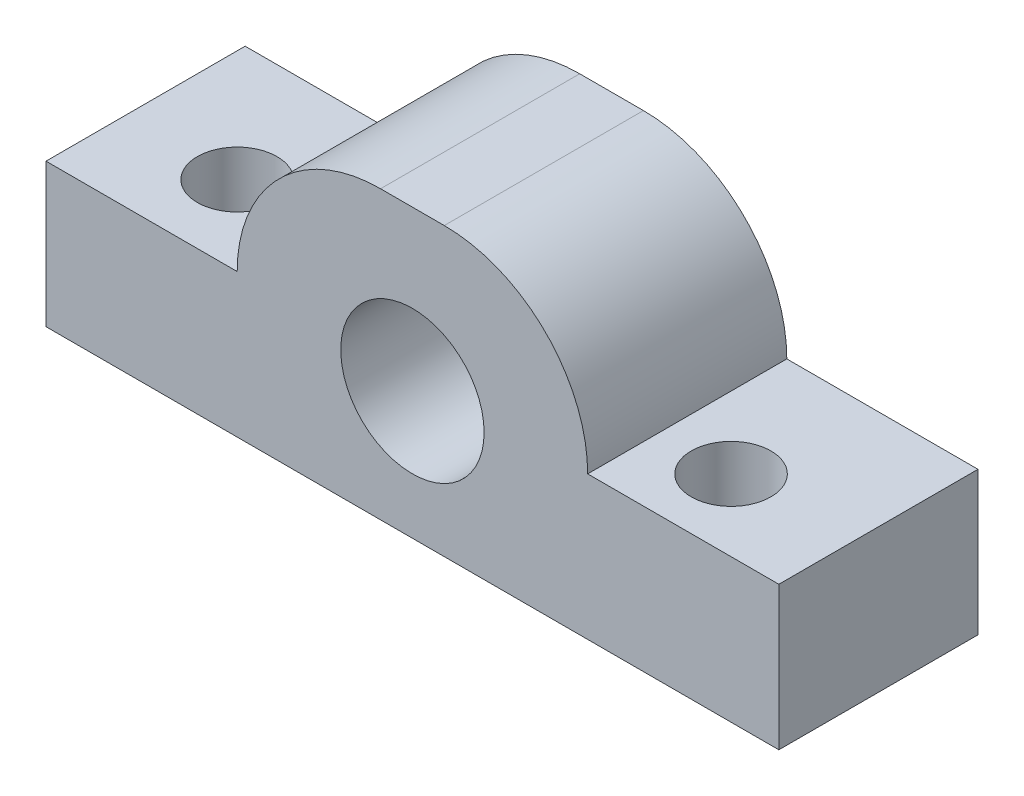
ISO-10303-21;
HEADER;
FILE_DESCRIPTION(('STEP AP214'),'2;1');
FILE_NAME('part.step','',(''),(''),'','','');
FILE_SCHEMA(('AUTOMOTIVE_DESIGN { 1 0 10303 214 1 1 1 1 }'));
ENDSEC;
DATA;
#1=APPLICATION_CONTEXT('core data for automotive mechanical design processes');
#2=APPLICATION_PROTOCOL_DEFINITION('international standard','automotive_design',2000,#1);
#3=PRODUCT_CONTEXT('',#1,'mechanical');
#4=PRODUCT('Part','Part','',(#3));
#5=PRODUCT_RELATED_PRODUCT_CATEGORY('part','',(#4));
#6=PRODUCT_DEFINITION_FORMATION('','',#4);
#7=PRODUCT_DEFINITION_CONTEXT('part definition',#1,'design');
#8=PRODUCT_DEFINITION('design','',#6,#7);
#9=PRODUCT_DEFINITION_SHAPE('','',#8);
#10=(LENGTH_UNIT() NAMED_UNIT(*) SI_UNIT(.MILLI.,.METRE.));
#11=(NAMED_UNIT(*) PLANE_ANGLE_UNIT() SI_UNIT($,.RADIAN.));
#12=(NAMED_UNIT(*) SI_UNIT($,.STERADIAN.) SOLID_ANGLE_UNIT());
#13=UNCERTAINTY_MEASURE_WITH_UNIT(LENGTH_MEASURE(1.E-05),#10,'distance_accuracy_value','');
#14=(GEOMETRIC_REPRESENTATION_CONTEXT(3) GLOBAL_UNCERTAINTY_ASSIGNED_CONTEXT((#13)) GLOBAL_UNIT_ASSIGNED_CONTEXT((#10,
#11,#12)) REPRESENTATION_CONTEXT('',''));
#15=CARTESIAN_POINT('',(0.,0.,0.));
#16=DIRECTION('',(0.,0.,1.));
#17=DIRECTION('',(1.,0.,0.));
#18=AXIS2_PLACEMENT_3D('',#15,#16,#17);
#19=CARTESIAN_POINT('',(-4.,18.,12.5));
#20=DIRECTION('',(0.,0.,-1.));
#21=DIRECTION('',(-1.,0.,0.));
#22=AXIS2_PLACEMENT_3D('',#19,#20,#21);
#23=PLANE('',#22);
#24=DIRECTION('',(0.,-1.,0.));
#25=VECTOR('',#24,1.);
#26=CARTESIAN_POINT('',(-46.,0.,12.5));
#27=LINE('',#26,#25);
#28=CARTESIAN_POINT('',(-46.,18.,12.5));
#29=VERTEX_POINT('',#28);
#30=CARTESIAN_POINT('',(-46.,0.,12.5));
#31=VERTEX_POINT('',#30);
#32=EDGE_CURVE('E151',#29,#31,#27,.T.);
#33=ORIENTED_EDGE('',*,*,#32,.T.);
#34=DIRECTION('',(1.,0.,0.));
#35=VECTOR('',#34,1.);
#36=CARTESIAN_POINT('',(46.,0.,12.5));
#37=LINE('',#36,#35);
#38=CARTESIAN_POINT('',(46.,0.,12.5));
#39=VERTEX_POINT('',#38);
#40=EDGE_CURVE('E97',#31,#39,#37,.T.);
#41=ORIENTED_EDGE('',*,*,#40,.T.);
#42=DIRECTION('',(0.,1.,0.));
#43=VECTOR('',#42,1.);
#44=CARTESIAN_POINT('',(46.,0.,12.5));
#45=LINE('',#44,#43);
#46=CARTESIAN_POINT('',(46.,18.,12.5));
#47=VERTEX_POINT('',#46);
#48=EDGE_CURVE('E167',#39,#47,#45,.T.);
#49=ORIENTED_EDGE('',*,*,#48,.T.);
#50=DIRECTION('',(-1.,0.,0.));
#51=VECTOR('',#50,1.);
#52=CARTESIAN_POINT('',(46.,18.,12.5));
#53=LINE('',#52,#51);
#54=CARTESIAN_POINT('',(22.,18.,12.5));
#55=VERTEX_POINT('',#54);
#56=EDGE_CURVE('E179',#47,#55,#53,.T.);
#57=ORIENTED_EDGE('',*,*,#56,.T.);
#58=CARTESIAN_POINT('',(4.,18.,12.5));
#59=DIRECTION('',(0.,0.,1.));
#60=DIRECTION('',(1.,0.,0.));
#61=AXIS2_PLACEMENT_3D('',#58,#59,#60);
#62=CIRCLE('',#61,18.);
#63=CARTESIAN_POINT('',(4.,36.,12.5));
#64=VERTEX_POINT('',#63);
#65=EDGE_CURVE('E120',#55,#64,#62,.T.);
#66=ORIENTED_EDGE('',*,*,#65,.T.);
#67=DIRECTION('',(-1.,0.,0.));
#68=VECTOR('',#67,1.);
#69=CARTESIAN_POINT('',(-4.,36.,12.5));
#70=LINE('',#69,#68);
#71=CARTESIAN_POINT('',(-4.,36.,12.5));
#72=VERTEX_POINT('',#71);
#73=EDGE_CURVE('E115',#64,#72,#70,.T.);
#74=ORIENTED_EDGE('',*,*,#73,.T.);
#75=CARTESIAN_POINT('',(-4.,18.,12.5));
#76=DIRECTION('',(0.,0.,1.));
#77=DIRECTION('',(-1.,0.,0.));
#78=AXIS2_PLACEMENT_3D('',#75,#76,#77);
#79=CIRCLE('',#78,18.);
#80=CARTESIAN_POINT('',(-22.,18.,12.5));
#81=VERTEX_POINT('',#80);
#82=EDGE_CURVE('E119',#72,#81,#79,.T.);
#83=ORIENTED_EDGE('',*,*,#82,.T.);
#84=DIRECTION('',(-1.,0.,0.));
#85=VECTOR('',#84,1.);
#86=CARTESIAN_POINT('',(-46.,18.,12.5));
#87=LINE('',#86,#85);
#88=EDGE_CURVE('E57',#81,#29,#87,.T.);
#89=ORIENTED_EDGE('',*,*,#88,.T.);
#90=EDGE_LOOP('',(#33,#41,#49,#57,#66,#74,#83,#89));
#91=FACE_BOUND('',#90,.T.);
#92=CARTESIAN_POINT('',(0.,16.,12.5));
#93=DIRECTION('',(0.,0.,1.));
#94=DIRECTION('',(1.,0.,0.));
#95=AXIS2_PLACEMENT_3D('',#92,#93,#94);
#96=CIRCLE('',#95,9.);
#97=CARTESIAN_POINT('',(9.,16.,12.5));
#98=VERTEX_POINT('',#97);
#99=EDGE_CURVE('E136',#98,#98,#96,.T.);
#100=ORIENTED_EDGE('',*,*,#99,.F.);
#101=EDGE_LOOP('',(#100));
#102=FACE_BOUND('',#101,.T.);
#103=ADVANCED_FACE('F39',(#91,#102),#23,.F.);
#104=CARTESIAN_POINT('',(-4.,18.,-12.5));
#105=DIRECTION('',(0.,0.,-1.));
#106=DIRECTION('',(-1.,0.,0.));
#107=AXIS2_PLACEMENT_3D('',#104,#105,#106);
#108=PLANE('',#107);
#109=DIRECTION('',(0.,-1.,0.));
#110=VECTOR('',#109,1.);
#111=CARTESIAN_POINT('',(-46.,0.,-12.5));
#112=LINE('',#111,#110);
#113=CARTESIAN_POINT('',(-46.,18.,-12.5));
#114=VERTEX_POINT('',#113);
#115=CARTESIAN_POINT('',(-46.,0.,-12.5));
#116=VERTEX_POINT('',#115);
#117=EDGE_CURVE('E137',#114,#116,#112,.T.);
#118=ORIENTED_EDGE('',*,*,#117,.F.);
#119=DIRECTION('',(-1.,0.,0.));
#120=VECTOR('',#119,1.);
#121=CARTESIAN_POINT('',(-46.,18.,-12.5));
#122=LINE('',#121,#120);
#123=CARTESIAN_POINT('',(-22.,18.,-12.5));
#124=VERTEX_POINT('',#123);
#125=EDGE_CURVE('E93',#124,#114,#122,.T.);
#126=ORIENTED_EDGE('',*,*,#125,.F.);
#127=CARTESIAN_POINT('',(-4.,18.,-12.5));
#128=DIRECTION('',(0.,0.,1.));
#129=DIRECTION('',(-1.,0.,0.));
#130=AXIS2_PLACEMENT_3D('',#127,#128,#129);
#131=CIRCLE('',#130,18.);
#132=CARTESIAN_POINT('',(-4.,36.,-12.5));
#133=VERTEX_POINT('',#132);
#134=EDGE_CURVE('E81',#133,#124,#131,.T.);
#135=ORIENTED_EDGE('',*,*,#134,.F.);
#136=DIRECTION('',(-1.,0.,0.));
#137=VECTOR('',#136,1.);
#138=CARTESIAN_POINT('',(-4.,36.,-12.5));
#139=LINE('',#138,#137);
#140=CARTESIAN_POINT('',(4.,36.,-12.5));
#141=VERTEX_POINT('',#140);
#142=EDGE_CURVE('E127',#141,#133,#139,.T.);
#143=ORIENTED_EDGE('',*,*,#142,.F.);
#144=CARTESIAN_POINT('',(4.,18.,-12.5));
#145=DIRECTION('',(0.,0.,1.));
#146=DIRECTION('',(1.,0.,0.));
#147=AXIS2_PLACEMENT_3D('',#144,#145,#146);
#148=CIRCLE('',#147,18.);
#149=CARTESIAN_POINT('',(22.,18.,-12.5));
#150=VERTEX_POINT('',#149);
#151=EDGE_CURVE('E148',#150,#141,#148,.T.);
#152=ORIENTED_EDGE('',*,*,#151,.F.);
#153=DIRECTION('',(-1.,0.,0.));
#154=VECTOR('',#153,1.);
#155=CARTESIAN_POINT('',(46.,18.,-12.5));
#156=LINE('',#155,#154);
#157=CARTESIAN_POINT('',(46.,18.,-12.5));
#158=VERTEX_POINT('',#157);
#159=EDGE_CURVE('E145',#158,#150,#156,.T.);
#160=ORIENTED_EDGE('',*,*,#159,.F.);
#161=DIRECTION('',(0.,1.,0.));
#162=VECTOR('',#161,1.);
#163=CARTESIAN_POINT('',(46.,0.,-12.5));
#164=LINE('',#163,#162);
#165=CARTESIAN_POINT('',(46.,0.,-12.5));
#166=VERTEX_POINT('',#165);
#167=EDGE_CURVE('E142',#166,#158,#164,.T.);
#168=ORIENTED_EDGE('',*,*,#167,.F.);
#169=DIRECTION('',(1.,0.,0.));
#170=VECTOR('',#169,1.);
#171=CARTESIAN_POINT('',(46.,0.,-12.5));
#172=LINE('',#171,#170);
#173=EDGE_CURVE('E139',#116,#166,#172,.T.);
#174=ORIENTED_EDGE('',*,*,#173,.F.);
#175=EDGE_LOOP('',(#118,#126,#135,#143,#152,#160,#168,#174));
#176=FACE_BOUND('',#175,.T.);
#177=CARTESIAN_POINT('',(0.,16.,-12.5));
#178=DIRECTION('',(0.,0.,1.));
#179=DIRECTION('',(1.,0.,0.));
#180=AXIS2_PLACEMENT_3D('',#177,#178,#179);
#181=CIRCLE('',#180,9.);
#182=CARTESIAN_POINT('',(9.,16.,-12.5));
#183=VERTEX_POINT('',#182);
#184=EDGE_CURVE('E183',#183,#183,#181,.T.);
#185=ORIENTED_EDGE('',*,*,#184,.T.);
#186=EDGE_LOOP('',(#185));
#187=FACE_BOUND('',#186,.T.);
#188=ADVANCED_FACE('F168',(#176,#187),#108,.T.);
#189=CARTESIAN_POINT('',(-46.,0.,12.5));
#190=DIRECTION('',(1.,0.,0.));
#191=DIRECTION('',(0.,0.,-1.));
#192=AXIS2_PLACEMENT_3D('',#189,#190,#191);
#193=PLANE('',#192);
#194=ORIENTED_EDGE('',*,*,#117,.T.);
#195=DIRECTION('',(0.,0.,-1.));
#196=VECTOR('',#195,1.);
#197=CARTESIAN_POINT('',(-46.,0.,12.5));
#198=LINE('',#197,#196);
#199=EDGE_CURVE('E11',#31,#116,#198,.T.);
#200=ORIENTED_EDGE('',*,*,#199,.F.);
#201=ORIENTED_EDGE('',*,*,#32,.F.);
#202=DIRECTION('',(0.,0.,-1.));
#203=VECTOR('',#202,1.);
#204=CARTESIAN_POINT('',(-46.,18.,12.5));
#205=LINE('',#204,#203);
#206=EDGE_CURVE('E131',#29,#114,#205,.T.);
#207=ORIENTED_EDGE('',*,*,#206,.T.);
#208=EDGE_LOOP('',(#194,#200,#201,#207));
#209=FACE_BOUND('',#208,.T.);
#210=ADVANCED_FACE('F41',(#209),#193,.F.);
#211=CARTESIAN_POINT('',(46.,0.,12.5));
#212=DIRECTION('',(0.,1.,0.));
#213=DIRECTION('',(0.,0.,1.));
#214=AXIS2_PLACEMENT_3D('',#211,#212,#213);
#215=PLANE('',#214);
#216=CARTESIAN_POINT('',(-32.,0.,2.5));
#217=DIRECTION('',(0.,1.,0.));
#218=DIRECTION('',(0.,0.,1.));
#219=AXIS2_PLACEMENT_3D('',#216,#217,#218);
#220=CIRCLE('',#219,5.);
#221=CARTESIAN_POINT('',(-32.,0.,7.5));
#222=VERTEX_POINT('',#221);
#223=EDGE_CURVE('E198',#222,#222,#220,.T.);
#224=ORIENTED_EDGE('',*,*,#223,.T.);
#225=EDGE_LOOP('',(#224));
#226=FACE_BOUND('',#225,.T.);
#227=CARTESIAN_POINT('',(31.,0.,3.5));
#228=DIRECTION('',(0.,1.,0.));
#229=DIRECTION('',(0.,0.,1.));
#230=AXIS2_PLACEMENT_3D('',#227,#228,#229);
#231=CIRCLE('',#230,5.);
#232=CARTESIAN_POINT('',(31.,0.,8.5));
#233=VERTEX_POINT('',#232);
#234=EDGE_CURVE('E190',#233,#233,#231,.T.);
#235=ORIENTED_EDGE('',*,*,#234,.T.);
#236=EDGE_LOOP('',(#235));
#237=FACE_BOUND('',#236,.T.);
#238=ORIENTED_EDGE('',*,*,#173,.T.);
#239=DIRECTION('',(0.,0.,-1.));
#240=VECTOR('',#239,1.);
#241=CARTESIAN_POINT('',(46.,0.,12.5));
#242=LINE('',#241,#240);
#243=EDGE_CURVE('E48',#39,#166,#242,.T.);
#244=ORIENTED_EDGE('',*,*,#243,.F.);
#245=ORIENTED_EDGE('',*,*,#40,.F.);
#246=ORIENTED_EDGE('',*,*,#199,.T.);
#247=EDGE_LOOP('',(#238,#244,#245,#246));
#248=FACE_BOUND('',#247,.T.);
#249=ADVANCED_FACE('F234',(#226,#237,#248),#215,.F.);
#250=CARTESIAN_POINT('',(46.,0.,12.5));
#251=DIRECTION('',(-1.,0.,0.));
#252=DIRECTION('',(0.,0.,1.));
#253=AXIS2_PLACEMENT_3D('',#250,#251,#252);
#254=PLANE('',#253);
#255=ORIENTED_EDGE('',*,*,#167,.T.);
#256=DIRECTION('',(0.,0.,-1.));
#257=VECTOR('',#256,1.);
#258=CARTESIAN_POINT('',(46.,18.,12.5));
#259=LINE('',#258,#257);
#260=EDGE_CURVE('E158',#47,#158,#259,.T.);
#261=ORIENTED_EDGE('',*,*,#260,.F.);
#262=ORIENTED_EDGE('',*,*,#48,.F.);
#263=ORIENTED_EDGE('',*,*,#243,.T.);
#264=EDGE_LOOP('',(#255,#261,#262,#263));
#265=FACE_BOUND('',#264,.T.);
#266=ADVANCED_FACE('F163',(#265),#254,.F.);
#267=CARTESIAN_POINT('',(46.,18.,12.5));
#268=DIRECTION('',(0.,-1.,0.));
#269=DIRECTION('',(1.,0.,0.));
#270=AXIS2_PLACEMENT_3D('',#267,#268,#269);
#271=PLANE('',#270);
#272=CARTESIAN_POINT('',(31.,18.,3.5));
#273=DIRECTION('',(0.,1.,0.));
#274=DIRECTION('',(0.,0.,1.));
#275=AXIS2_PLACEMENT_3D('',#272,#273,#274);
#276=CIRCLE('',#275,5.);
#277=CARTESIAN_POINT('',(31.,18.,8.5));
#278=VERTEX_POINT('',#277);
#279=EDGE_CURVE('E193',#278,#278,#276,.T.);
#280=ORIENTED_EDGE('',*,*,#279,.F.);
#281=EDGE_LOOP('',(#280));
#282=FACE_BOUND('',#281,.T.);
#283=ORIENTED_EDGE('',*,*,#159,.T.);
#284=DIRECTION('',(0.,0.,-1.));
#285=VECTOR('',#284,1.);
#286=CARTESIAN_POINT('',(22.,18.,12.5));
#287=LINE('',#286,#285);
#288=EDGE_CURVE('E154',#55,#150,#287,.T.);
#289=ORIENTED_EDGE('',*,*,#288,.F.);
#290=ORIENTED_EDGE('',*,*,#56,.F.);
#291=ORIENTED_EDGE('',*,*,#260,.T.);
#292=EDGE_LOOP('',(#283,#289,#290,#291));
#293=FACE_BOUND('',#292,.T.);
#294=ADVANCED_FACE('F172',(#282,#293),#271,.F.);
#295=CARTESIAN_POINT('',(4.,18.,12.5));
#296=DIRECTION('',(0.,0.,-1.));
#297=DIRECTION('',(-1.,0.,0.));
#298=AXIS2_PLACEMENT_3D('',#295,#296,#297);
#299=CYLINDRICAL_SURFACE('',#298,18.);
#300=ORIENTED_EDGE('',*,*,#151,.T.);
#301=DIRECTION('',(0.,0.,-1.));
#302=VECTOR('',#301,1.);
#303=CARTESIAN_POINT('',(4.,36.,12.5));
#304=LINE('',#303,#302);
#305=EDGE_CURVE('E130',#64,#141,#304,.T.);
#306=ORIENTED_EDGE('',*,*,#305,.F.);
#307=ORIENTED_EDGE('',*,*,#65,.F.);
#308=ORIENTED_EDGE('',*,*,#288,.T.);
#309=EDGE_LOOP('',(#300,#306,#307,#308));
#310=FACE_BOUND('',#309,.T.);
#311=ADVANCED_FACE('F178',(#310),#299,.T.);
#312=CARTESIAN_POINT('',(-4.,36.,12.5));
#313=DIRECTION('',(0.,-1.,0.));
#314=DIRECTION('',(0.,0.,-1.));
#315=AXIS2_PLACEMENT_3D('',#312,#313,#314);
#316=PLANE('',#315);
#317=ORIENTED_EDGE('',*,*,#142,.T.);
#318=DIRECTION('',(0.,0.,-1.));
#319=VECTOR('',#318,1.);
#320=CARTESIAN_POINT('',(-4.,36.,12.5));
#321=LINE('',#320,#319);
#322=EDGE_CURVE('E123',#72,#133,#321,.T.);
#323=ORIENTED_EDGE('',*,*,#322,.F.);
#324=ORIENTED_EDGE('',*,*,#73,.F.);
#325=ORIENTED_EDGE('',*,*,#305,.T.);
#326=EDGE_LOOP('',(#317,#323,#324,#325));
#327=FACE_BOUND('',#326,.T.);
#328=ADVANCED_FACE('F124',(#327),#316,.F.);
#329=CARTESIAN_POINT('',(-4.,18.,12.5));
#330=DIRECTION('',(0.,0.,-1.));
#331=DIRECTION('',(-1.,0.,0.));
#332=AXIS2_PLACEMENT_3D('',#329,#330,#331);
#333=CYLINDRICAL_SURFACE('',#332,18.);
#334=ORIENTED_EDGE('',*,*,#134,.T.);
#335=DIRECTION('',(0.,0.,-1.));
#336=VECTOR('',#335,1.);
#337=CARTESIAN_POINT('',(-22.,18.,12.5));
#338=LINE('',#337,#336);
#339=EDGE_CURVE('E126',#81,#124,#338,.T.);
#340=ORIENTED_EDGE('',*,*,#339,.F.);
#341=ORIENTED_EDGE('',*,*,#82,.F.);
#342=ORIENTED_EDGE('',*,*,#322,.T.);
#343=EDGE_LOOP('',(#334,#340,#341,#342));
#344=FACE_BOUND('',#343,.T.);
#345=ADVANCED_FACE('F128',(#344),#333,.T.);
#346=CARTESIAN_POINT('',(-46.,18.,12.5));
#347=DIRECTION('',(0.,-1.,0.));
#348=DIRECTION('',(1.,0.,0.));
#349=AXIS2_PLACEMENT_3D('',#346,#347,#348);
#350=PLANE('',#349);
#351=CARTESIAN_POINT('',(-32.,18.,2.5));
#352=DIRECTION('',(0.,1.,0.));
#353=DIRECTION('',(0.,0.,1.));
#354=AXIS2_PLACEMENT_3D('',#351,#352,#353);
#355=CIRCLE('',#354,5.);
#356=CARTESIAN_POINT('',(-32.,18.,7.5));
#357=VERTEX_POINT('',#356);
#358=EDGE_CURVE('E200',#357,#357,#355,.T.);
#359=ORIENTED_EDGE('',*,*,#358,.F.);
#360=EDGE_LOOP('',(#359));
#361=FACE_BOUND('',#360,.T.);
#362=ORIENTED_EDGE('',*,*,#125,.T.);
#363=ORIENTED_EDGE('',*,*,#206,.F.);
#364=ORIENTED_EDGE('',*,*,#88,.F.);
#365=ORIENTED_EDGE('',*,*,#339,.T.);
#366=EDGE_LOOP('',(#362,#363,#364,#365));
#367=FACE_BOUND('',#366,.T.);
#368=ADVANCED_FACE('F202',(#361,#367),#350,.F.);
#369=CARTESIAN_POINT('',(0.,16.,12.5));
#370=DIRECTION('',(0.,0.,-1.));
#371=DIRECTION('',(-1.,0.,0.));
#372=AXIS2_PLACEMENT_3D('',#369,#370,#371);
#373=CYLINDRICAL_SURFACE('',#372,9.);
#374=ORIENTED_EDGE('',*,*,#99,.T.);
#375=EDGE_LOOP('',(#374));
#376=FACE_BOUND('',#375,.T.);
#377=ORIENTED_EDGE('',*,*,#184,.F.);
#378=EDGE_LOOP('',(#377));
#379=FACE_BOUND('',#378,.T.);
#380=ADVANCED_FACE('F210',(#376,#379),#373,.F.);
#381=CARTESIAN_POINT('',(31.,18.,3.5));
#382=DIRECTION('',(0.,1.,0.));
#383=DIRECTION('',(0.,0.,1.));
#384=AXIS2_PLACEMENT_3D('',#381,#382,#383);
#385=CYLINDRICAL_SURFACE('',#384,5.);
#386=ORIENTED_EDGE('',*,*,#234,.F.);
#387=EDGE_LOOP('',(#386));
#388=FACE_BOUND('',#387,.T.);
#389=ORIENTED_EDGE('',*,*,#279,.T.);
#390=EDGE_LOOP('',(#389));
#391=FACE_BOUND('',#390,.T.);
#392=ADVANCED_FACE('F212',(#388,#391),#385,.F.);
#393=CARTESIAN_POINT('',(-32.,18.,2.5));
#394=DIRECTION('',(0.,1.,0.));
#395=DIRECTION('',(0.,0.,1.));
#396=AXIS2_PLACEMENT_3D('',#393,#394,#395);
#397=CYLINDRICAL_SURFACE('',#396,5.);
#398=ORIENTED_EDGE('',*,*,#223,.F.);
#399=EDGE_LOOP('',(#398));
#400=FACE_BOUND('',#399,.T.);
#401=ORIENTED_EDGE('',*,*,#358,.T.);
#402=EDGE_LOOP('',(#401));
#403=FACE_BOUND('',#402,.T.);
#404=ADVANCED_FACE('F201',(#400,#403),#397,.F.);
#405=CLOSED_SHELL('',(#103,#188,#210,#249,#266,#294,#311,#328,#345,#368,#380,#392,#404));
#406=MANIFOLD_SOLID_BREP('B2',#405);
#407=ADVANCED_BREP_SHAPE_REPRESENTATION('',(#18,#406),#14);
#408=SHAPE_DEFINITION_REPRESENTATION(#9,#407);
ENDSEC;
END-ISO-10303-21;
